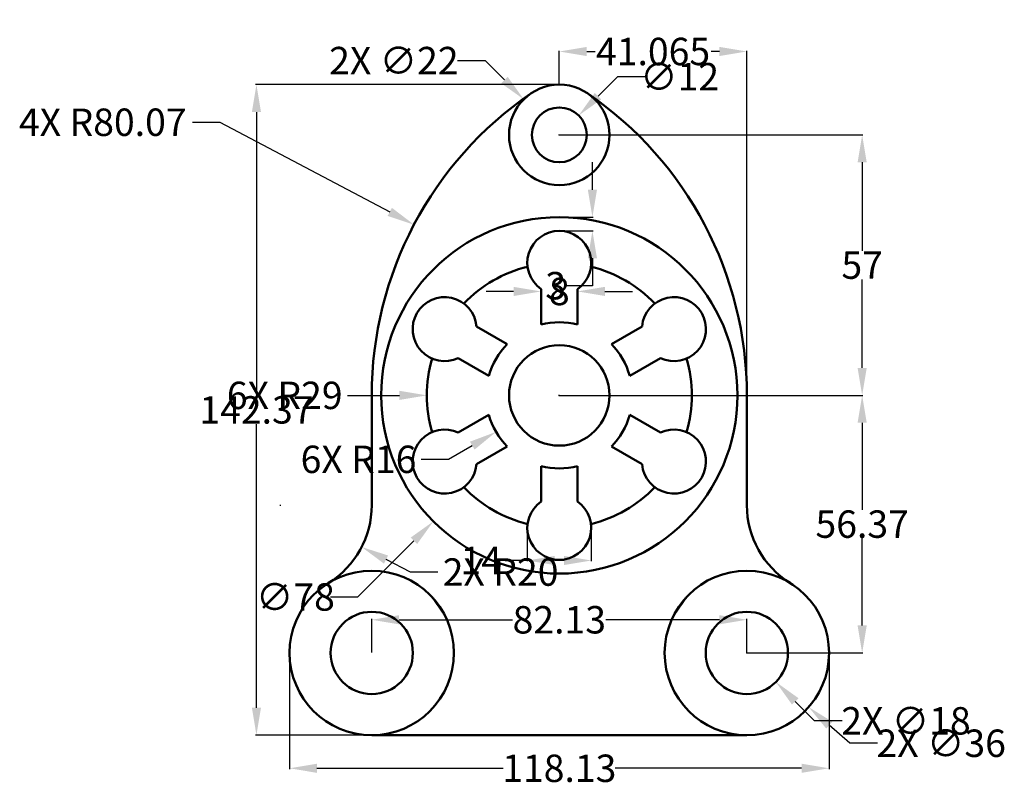
# Model space of a CAD drawing. Units: millimetres. Extents: x 708 to 923, y 97 to 265.
import ezdxf

# ---------------------------------------------------------------- set-up
doc = ezdxf.new("R2010")
doc.units = ezdxf.units.MM
doc.header["$MEASUREMENT"] = 0
doc.layers.add('M-DIMS', color=2, linetype='Continuous', lineweight=18)
doc.layers.add('M-OUTL', color=7, linetype='Continuous', lineweight=50)
doc.styles.get("Standard").update_dxf_attribs({"font": 'arial.ttf'})
doc.dimstyles.get("Standard").update_dxf_attribs({"dimtxt": 6, "dimasz": 6, "dimexe": 0.18, "dimexo": 0.0625, "dimgap": 0.09, "dimtad": 0, "dimtih": 1, "dimtoh": 1, "dimdec": 0, "dimzin": 0, "dimdsep": 46, "dimtxsty": 'Standard', "dimcen": 0.09, "dimadec": 0, "dimazin": 0, "dimtfac": 1, "dimtdec": 0, "dimtofl": 0, "dimtmove": 0, "dimatfit": 3, "dimfxl": 1, "dimtolj": 1, "dimtzin": 0, "dimarcsym": 0})

# ---------------------------------------------------------------- blocks, each defined once
blk = doc.blocks.new('*U1')
for p, q in [((-4, -10.25), (-4, -2.49)), ((4, -10.25), (4, -2.49))]:
    blk.add_line(p, q)
blk.add_arc((0, 3.25), 7, 304.8499, 235.1501)
blk = doc.blocks.new('*U2')
at = {"layer": 'M-OUTL', "color": 0, "linetype": 'ByBlock', "lineweight": -2, "transparency": 16777216}
blk.add_blockref('*U1', (825.86, 208.55), dxfattribs=at)
for p, rotation in [((803.57, 195.67), 60), ((848.16, 195.67), 300), ((803.57, 169.93), 120), ((848.16, 169.93), 240), ((825.86, 157.05), 180)]:
    blk.add_blockref('*U1', p, dxfattribs=dict(at, rotation=rotation))
blk = doc.blocks.new('MOUNTING-EAR-OD36-BORE18')
for radius in [18, 9]:
    blk.add_circle((0, 0), radius)
blk = doc.blocks.new('*D4')
at = {"layer": 'Defpoints', "color": 0, "transparency": 16777216}
for p in [(766.8, 126.44), (884.93, 126.44), (884.93, 101.19)]:
    blk.add_point(p, dxfattribs=at)
at = {"layer": 'M-DIMS', "color": 0, "lineweight": -2, "transparency": 16777216}
for p, q in [((766.8, 126.37), (766.8, 101.01)), ((884.93, 126.37), (884.93, 101.01)), ((772.8, 101.19), (813.6, 101.19)), ((878.93, 101.19), (838.13, 101.19))]:
    blk.add_line(p, q, dxfattribs=at)
at = {"layer": 'M-DIMS', "color": 0, "transparency": 16777216}
for points in [[(772.8, 102.19), (772.8, 100.19), (766.8, 101.19)], [(878.93, 102.19), (878.93, 100.19), (884.93, 101.19)]]:
    blk.add_solid(points, dxfattribs=at)
at = {"layer": 'M-DIMS', "color": 0, "transparency": 16777216, "insert": (825.86, 101.19), "char_height": 6, "attachment_point": 5}
blk.add_mtext('\\A1;118.13', dxfattribs=at)
blk = doc.blocks.new('*D5')
at = {"layer": 'Defpoints', "color": 0, "transparency": 16777216}
for p in [(759.55, 250.8), (825.86, 250.8), (784.8, 108.44)]:
    blk.add_point(p, dxfattribs=at)
at = {"layer": 'M-DIMS', "color": 0, "lineweight": -2, "transparency": 16777216}
for p, q in [((825.8, 250.8), (759.37, 250.8)), ((759.55, 244.8), (759.55, 182.77)), ((759.55, 114.44), (759.55, 176.46)), ((784.74, 108.44), (759.37, 108.44))]:
    blk.add_line(p, q, dxfattribs=at)
at = {"layer": 'M-DIMS', "color": 0, "transparency": 16777216}
for points in [[(758.55, 244.8), (760.55, 244.8), (759.55, 250.8)], [(758.55, 114.44), (760.55, 114.44), (759.55, 108.44)]]:
    blk.add_solid(points, dxfattribs=at)
at = {"layer": 'M-DIMS', "color": 0, "transparency": 16777216, "insert": (759.55, 179.62), "char_height": 6, "attachment_point": 5}
blk.add_mtext('\\A1;142.37', dxfattribs=at)
blk = doc.blocks.new('*D6')
at = {"layer": 'Defpoints', "color": 0, "transparency": 16777216}
for p in [(825.86, 182.8), (892.18, 182.8), (866.93, 126.44)]:
    blk.add_point(p, dxfattribs=at)
at = {"layer": 'M-DIMS', "color": 0, "lineweight": -2, "transparency": 16777216}
for p, q in [((825.93, 182.8), (892.36, 182.8)), ((892.18, 176.8), (892.18, 157.77)), ((892.18, 132.44), (892.18, 151.46)), ((866.99, 126.44), (892.36, 126.44))]:
    blk.add_line(p, q, dxfattribs=at)
at = {"layer": 'M-DIMS', "color": 0, "transparency": 16777216}
for points in [[(891.18, 176.8), (893.18, 176.8), (892.18, 182.8)], [(891.18, 132.44), (893.18, 132.44), (892.18, 126.44)]]:
    blk.add_solid(points, dxfattribs=at)
at = {"layer": 'M-DIMS', "color": 0, "transparency": 16777216, "insert": (892.18, 154.62), "char_height": 6, "attachment_point": 5}
blk.add_mtext('\\A1;56.37', dxfattribs=at)
blk = doc.blocks.new('*D7')
at = {"layer": 'Defpoints', "color": 0, "transparency": 16777216}
for p in [(825.86, 239.8), (892.18, 239.8), (866.93, 182.8)]:
    blk.add_point(p, dxfattribs=at)
at = {"layer": 'M-DIMS', "color": 0, "lineweight": -2, "transparency": 16777216}
for p, q in [((825.93, 239.8), (892.36, 239.8)), ((892.18, 233.8), (892.18, 214.44)), ((892.18, 188.8), (892.18, 208.16)), ((866.99, 182.8), (892.36, 182.8))]:
    blk.add_line(p, q, dxfattribs=at)
at = {"layer": 'M-DIMS', "color": 0, "transparency": 16777216}
for points in [[(891.18, 233.8), (893.18, 233.8), (892.18, 239.8)], [(891.18, 188.8), (893.18, 188.8), (892.18, 182.8)]]:
    blk.add_solid(points, dxfattribs=at)
at = {"layer": 'M-DIMS', "color": 0, "transparency": 16777216, "insert": (892.18, 211.3), "char_height": 6, "attachment_point": 5}
blk.add_mtext('\\A1;57', dxfattribs=at)
blk = doc.blocks.new('*D8')
at = {"layer": 'Defpoints', "color": 0, "transparency": 16777216}
for p in [(866.93, 133.69), (784.8, 126.44), (866.93, 126.44)]:
    blk.add_point(p, dxfattribs=at)
at = {"layer": 'M-DIMS', "color": 0, "lineweight": -2, "transparency": 16777216}
for p, q in [((784.8, 126.5), (784.8, 133.87)), ((790.8, 133.69), (815.65, 133.69)), ((860.93, 133.69), (836.08, 133.69)), ((866.93, 126.5), (866.93, 133.87))]:
    blk.add_line(p, q, dxfattribs=at)
at = {"layer": 'M-DIMS', "color": 0, "transparency": 16777216}
for points in [[(790.8, 134.69), (790.8, 132.69), (784.8, 133.69)], [(860.93, 134.69), (860.93, 132.69), (866.93, 133.69)]]:
    blk.add_solid(points, dxfattribs=at)
at = {"layer": 'M-DIMS', "color": 0, "transparency": 16777216, "insert": (825.86, 133.69), "char_height": 6, "attachment_point": 5}
blk.add_mtext('\\A1;82.13', dxfattribs=at)
blk = doc.blocks.new('*D9')
at = {"layer": 'Defpoints', "color": 0, "transparency": 16777216}
for p in [(866.93, 258.05), (825.86, 250.8), (866.93, 182.8)]:
    blk.add_point(p, dxfattribs=at)
at = {"layer": 'M-DIMS', "color": 0, "lineweight": -2, "transparency": 16777216}
for p, q in [((825.86, 250.86), (825.86, 258.23)), ((831.86, 258.05), (833.71, 258.05)), ((860.93, 258.05), (859.08, 258.05)), ((866.93, 182.86), (866.93, 258.23))]:
    blk.add_line(p, q, dxfattribs=at)
at = {"layer": 'M-DIMS', "color": 0, "transparency": 16777216}
for points in [[(831.86, 259.05), (831.86, 257.05), (825.86, 258.05)], [(860.93, 259.05), (860.93, 257.05), (866.93, 258.05)]]:
    blk.add_solid(points, dxfattribs=at)
at = {"layer": 'M-DIMS', "color": 0, "transparency": 16777216, "insert": (846.4, 258.05), "char_height": 6, "attachment_point": 5}
blk.add_mtext('\\A1;41.065', dxfattribs=at)
blk = doc.blocks.new('*D10')
at = {"layer": 'Defpoints', "color": 0, "transparency": 16777216}
for p in [(829.864092, 205.542651), (821.864092, 198.292651), (829.864092, 198.292651)]:
    blk.add_point(p, dxfattribs=at)
at = {"layer": 'M-DIMS', "color": 0, "lineweight": -2, "transparency": 16777216}
for p, q in [((815.864092, 205.542651), (809.864092, 205.542651)), ((821.864092, 198.355151), (821.864092, 205.722651)), ((829.864092, 198.355151), (829.864092, 205.722651)), ((835.864092, 205.542651), (841.864092, 205.542651))]:
    blk.add_line(p, q, dxfattribs=at)
at = {"layer": 'M-DIMS', "color": 0, "transparency": 16777216}
for points in [[(815.864092, 206.542651), (815.864092, 204.542651), (821.864092, 205.542651)], [(835.864092, 206.542651), (835.864092, 204.542651), (829.864092, 205.542651)]]:
    blk.add_solid(points, dxfattribs=at)
at = {"layer": 'M-DIMS', "color": 0, "transparency": 16777216, "insert": (825.864092, 205.542651), "char_height": 6, "attachment_point": 5}
blk.add_mtext('\\A1;8', dxfattribs=at)
blk = doc.blocks.new('*D11')
at = {"layer": 'Defpoints', "color": 0, "transparency": 16777216}
for p in [(818.86, 153.91), (832.86, 153.91), (818.86, 146.66)]:
    blk.add_point(p, dxfattribs=at)
at = {"layer": 'M-DIMS', "color": 0, "lineweight": -2, "transparency": 16777216}
for p, q in [((818.86, 153.85), (818.86, 146.48)), ((832.86, 153.85), (832.86, 146.48)), ((818.86, 146.66), (812.86, 146.66)), ((826.86, 146.66), (824.86, 146.66))]:
    blk.add_line(p, q, dxfattribs=at)
at = {"layer": 'M-DIMS', "color": 0, "transparency": 16777216}
for points in [[(824.86, 147.66), (824.86, 145.66), (818.86, 146.66)], [(826.86, 147.66), (826.86, 145.66), (832.86, 146.66)]]:
    blk.add_solid(points, dxfattribs=at)
at = {"layer": 'M-DIMS', "color": 0, "transparency": 16777216, "insert": (808.77, 146.66), "char_height": 6, "attachment_point": 5}
blk.add_mtext('\\A1;14', dxfattribs=at)
blk = doc.blocks.new('*D12')
at = {"layer": 'Defpoints', "color": 0, "transparency": 16777216}
for p in [(825.86, 221.8), (825.86, 218.8), (833.11, 218.8)]:
    blk.add_point(p, dxfattribs=at)
at = {"layer": 'M-DIMS', "color": 0, "lineweight": -2, "transparency": 16777216}
for p, q in [((833.11, 227.8), (833.11, 233.8)), ((825.93, 221.8), (833.29, 221.8)), ((825.93, 218.8), (833.29, 218.8)), ((833.11, 212.8), (833.11, 206.8)), ((833.11, 206.8), (827.11, 206.8))]:
    blk.add_line(p, q, dxfattribs=at)
at = {"layer": 'M-DIMS', "color": 0, "transparency": 16777216}
for points in [[(832.11, 227.8), (834.11, 227.8), (833.11, 221.8)], [(832.11, 212.8), (834.11, 212.8), (833.11, 218.8)]]:
    blk.add_solid(points, dxfattribs=at)
at = {"layer": 'M-DIMS', "color": 0, "transparency": 16777216, "insert": (825.06, 206.8), "char_height": 6, "attachment_point": 5}
blk.add_mtext('\\A1;3', dxfattribs=at)
blk = doc.blocks.new('*D13')
at = {"layer": 'Defpoints', "color": 0, "transparency": 16777216}
for p in [(853.39, 138.3), (880.47, 114.58)]:
    blk.add_point(p, dxfattribs=at)
at = {"layer": 'M-DIMS', "color": 0, "lineweight": -2, "transparency": 16777216}
for p, q in [((866.84, 126.44), (867.02, 126.44)), ((866.93, 126.35), (866.93, 126.53)), ((889.5, 106.67), (884.98, 110.62)), ((895.5, 106.67), (889.5, 106.67))]:
    blk.add_line(p, q, dxfattribs=at)
at = {"layer": 'M-DIMS', "color": 0, "transparency": 16777216}
blk.add_solid([(885.64, 111.38), (884.32, 109.87), (880.47, 114.58)], dxfattribs=at)
at = {"layer": 'M-DIMS', "color": 0, "transparency": 16777216, "insert": (909.48, 106.67), "char_height": 6, "attachment_point": 5}
blk.add_mtext('\\A1;2X ∅36', dxfattribs=at)
blk = doc.blocks.new('*D14')
at = {"layer": 'Defpoints', "color": 0, "transparency": 16777216}
for p in [(860.57, 132.8), (873.29, 120.07)]:
    blk.add_point(p, dxfattribs=at)
at = {"layer": 'M-DIMS', "color": 0, "lineweight": -2, "transparency": 16777216}
for p, q in [((866.84, 126.44), (867.02, 126.44)), ((866.93, 126.35), (866.93, 126.53)), ((881.77, 111.58), (877.53, 115.82)), ((887.77, 111.58), (881.77, 111.58))]:
    blk.add_line(p, q, dxfattribs=at)
at = {"layer": 'M-DIMS', "color": 0, "transparency": 16777216}
blk.add_solid([(878.24, 116.53), (876.82, 115.12), (873.29, 120.07)], dxfattribs=at)
at = {"layer": 'M-DIMS', "color": 0, "transparency": 16777216, "insert": (901.77, 111.58), "char_height": 6, "attachment_point": 5}
blk.add_mtext('\\A1;2X ∅18', dxfattribs=at)
blk = doc.blocks.new('*D15')
at = {"layer": 'Defpoints', "color": 0, "transparency": 16777216}
for p in [(830.11, 244.05), (821.62, 235.56)]:
    blk.add_point(p, dxfattribs=at)
at = {"layer": 'M-DIMS', "color": 0, "lineweight": -2, "transparency": 16777216}
for p, q in [((838.59, 252.53), (834.35, 248.29)), ((844.59, 252.53), (838.59, 252.53)), ((825.77, 239.8), (825.95, 239.8)), ((825.86, 239.71), (825.86, 239.89))]:
    blk.add_line(p, q, dxfattribs=at)
at = {"layer": 'M-DIMS', "color": 0, "transparency": 16777216}
blk.add_solid([(833.64, 249), (835.05, 247.58), (830.11, 244.05)], dxfattribs=at)
at = {"layer": 'M-DIMS', "color": 0, "transparency": 16777216, "insert": (852.21, 252.53), "char_height": 6, "attachment_point": 5}
blk.add_mtext('\\A1;∅12', dxfattribs=at)
blk = doc.blocks.new('*D16')
at = {"layer": 'Defpoints', "color": 0, "transparency": 16777216}
for p in [(818.08, 247.58), (833.64, 232.02)]:
    blk.add_point(p, dxfattribs=at)
at = {"layer": 'M-DIMS', "color": 0, "lineweight": -2, "transparency": 16777216}
for p, q in [((803.6, 256.06), (809.6, 256.06)), ((809.6, 256.06), (813.84, 251.82)), ((825.77, 239.8), (825.95, 239.8)), ((825.86, 239.71), (825.86, 239.89))]:
    blk.add_line(p, q, dxfattribs=at)
at = {"layer": 'M-DIMS', "color": 0, "transparency": 16777216}
blk.add_solid([(814.55, 252.53), (813.13, 251.11), (818.08, 247.58)], dxfattribs=at)
at = {"layer": 'M-DIMS', "color": 0, "transparency": 16777216, "insert": (789.64, 256.06), "char_height": 6, "attachment_point": 5}
blk.add_mtext('\\A1;2X ∅22', dxfattribs=at)
blk = doc.blocks.new('*D17')
at = {"layer": 'Defpoints', "color": 0, "transparency": 16777216}
for p in [(794.05, 220.15), (864.86, 182.8)]:
    blk.add_point(p, dxfattribs=at)
at = {"layer": 'M-DIMS', "color": 0, "lineweight": -2, "transparency": 16777216}
for p, q in [((745.56, 242.57), (751.56, 242.57)), ((751.56, 242.57), (788.74, 222.95)), ((864.77, 182.8), (864.95, 182.8)), ((864.86, 182.71), (864.86, 182.89))]:
    blk.add_line(p, q, dxfattribs=at)
at = {"layer": 'M-DIMS', "color": 0, "transparency": 16777216}
blk.add_solid([(789.21, 223.84), (788.27, 222.07), (794.05, 220.15)], dxfattribs=at)
at = {"layer": 'M-DIMS', "color": 0, "transparency": 16777216, "insert": (725.9, 242.57), "char_height": 6, "attachment_point": 5}
blk.add_mtext('\\A1;4X R80.07', dxfattribs=at)
blk = doc.blocks.new('*D18')
at = {"layer": 'Defpoints', "color": 0, "transparency": 16777216}
for p in [(764.8, 158.75), (782.59, 149.61)]:
    blk.add_point(p, dxfattribs=at)
at = {"layer": 'M-DIMS', "color": 0, "lineweight": -2, "transparency": 16777216}
for p, q in [((764.71, 158.75), (764.89, 158.75)), ((764.8, 158.66), (764.8, 158.84)), ((793.26, 144.13), (787.93, 146.87)), ((799.26, 144.13), (793.26, 144.13))]:
    blk.add_line(p, q, dxfattribs=at)
at = {"layer": 'M-DIMS', "color": 0, "transparency": 16777216}
blk.add_solid([(788.38, 147.76), (787.47, 145.98), (782.59, 149.61)], dxfattribs=at)
at = {"layer": 'M-DIMS', "color": 0, "transparency": 16777216, "insert": (813.01, 144.13), "char_height": 6, "attachment_point": 5}
blk.add_mtext('\\A1;2X R20', dxfattribs=at)
blk = doc.blocks.new('*D19')
at = {"layer": 'Defpoints', "color": 0, "transparency": 16777216}
for p in [(853.44, 210.38), (798.29, 155.22)]:
    blk.add_point(p, dxfattribs=at)
at = {"layer": 'M-DIMS', "color": 0, "lineweight": -2, "transparency": 16777216}
for p, q in [((825.77, 182.8), (825.95, 182.8)), ((825.86, 182.71), (825.86, 182.89)), ((781.74, 138.68), (794.04, 150.98)), ((775.74, 138.68), (781.74, 138.68))]:
    blk.add_line(p, q, dxfattribs=at)
at = {"layer": 'M-DIMS', "color": 0, "transparency": 16777216}
blk.add_solid([(793.34, 151.69), (794.75, 150.28), (798.29, 155.22)], dxfattribs=at)
at = {"layer": 'M-DIMS', "color": 0, "transparency": 16777216, "insert": (768.08, 138.68), "char_height": 6, "attachment_point": 5}
blk.add_mtext('\\A1;∅78', dxfattribs=at)
blk = doc.blocks.new('*D20')
at = {"layer": 'Defpoints', "color": 0, "transparency": 16777216}
for p in [(796.86, 182.8), (825.86, 182.8)]:
    blk.add_point(p, dxfattribs=at)
at = {"layer": 'M-DIMS', "color": 0, "lineweight": -2, "transparency": 16777216}
for p, q in [((779.46, 182.8), (790.86, 182.8)), ((825.77, 182.8), (825.95, 182.8)), ((825.86, 182.71), (825.86, 182.89))]:
    blk.add_line(p, q, dxfattribs=at)
at = {"layer": 'M-DIMS', "color": 0, "transparency": 16777216}
blk.add_solid([(790.86, 183.8), (790.86, 181.8), (796.86, 182.8)], dxfattribs=at)
at = {"layer": 'M-DIMS', "color": 0, "transparency": 16777216, "insert": (765.74, 182.8), "char_height": 6, "attachment_point": 5}
blk.add_mtext('\\A1;6X R29', dxfattribs=at)
blk = doc.blocks.new('*D21')
at = {"layer": 'Defpoints', "color": 0, "transparency": 16777216}
for p in [(825.86, 182.8), (812.01, 174.8)]:
    blk.add_point(p, dxfattribs=at)
at = {"layer": 'M-DIMS', "color": 0, "lineweight": -2, "transparency": 16777216}
for p, q in [((825.77, 182.8), (825.95, 182.8)), ((825.86, 182.71), (825.86, 182.89)), ((801.62, 168.8), (806.81, 171.8)), ((795.62, 168.8), (801.62, 168.8))]:
    blk.add_line(p, q, dxfattribs=at)
at = {"layer": 'M-DIMS', "color": 0, "transparency": 16777216}
blk.add_solid([(806.31, 172.67), (807.31, 170.93), (812.01, 174.8)], dxfattribs=at)
at = {"layer": 'M-DIMS', "color": 0, "transparency": 16777216, "insert": (781.9, 168.8), "char_height": 6, "attachment_point": 5}
blk.add_mtext('\\A1;6X R16', dxfattribs=at)

msp = doc.modelspace()

# ---------------------------------------------------------------- linework, layer by layer
at = {"layer": 'M-OUTL'}
for p, q in [((784.7989, 182.8007), (784.7989, 158.7466)), ((866.9293, 182.8007), (866.9293, 158.7466)), ((784.7989, 108.4357), (866.9293, 108.4357))]:
    msp.add_line(p, q, dxfattribs=at)
for centre, radius in [((825.8641, 239.8007), 11), ((825.8641, 239.8007), 6), ((825.8641, 182.8007), 39), ((825.8641, 182.8007), 11)]:
    msp.add_circle(centre, radius, dxfattribs=at)
for centre, radius, start, end in [((864.8641, 182.8007), 80.0652, 124.380345, 180), ((786.8641, 182.8007), 80.0652, 0, 55.619655), ((825.8641, 182.8007), 29, 103.863812, 136.136188), ((825.8641, 182.8007), 29, 43.863812, 76.136188), ((825.8641, 182.8007), 16, 75.522488, 104.477512), ((825.8641, 182.8007), 16, 135.522488, 164.477512), ((825.8641, 182.8007), 16, 15.522488, 44.477512), ((825.8641, 182.8007), 29, 163.863812, 196.136188), ((825.8641, 182.8007), 29, 343.863812, 16.136188), ((825.8641, 182.8007), 16, 195.522488, 224.477512), ((825.8641, 182.8007), 16, 315.522488, 344.477512), ((825.8641, 182.8007), 16, 255.522488, 284.477512), ((825.8641, 182.8007), 29, 223.863812, 256.136188), ((825.8641, 182.8007), 29, 283.863812, 316.136188), ((764.7989, 158.7466), 20, 301.756864, 0), ((886.9293, 158.7466), 20, 180, 238.243136), ((864.8641, 182.8007), 80.0652, 213.646297, 216.643999), ((786.8641, 182.8007), 80.0652, 323.356001, 326.353703)]:
    msp.add_arc(centre, radius, start, end, dxfattribs=at)

# ---------------------------------------------------------------- block references
for name, p in [('*U2', (0, 0)), ('MOUNTING-EAR-OD36-BORE18', (784.7989, 126.4357)), ('MOUNTING-EAR-OD36-BORE18', (866.9293, 126.4357))]:
    msp.add_blockref(name, p, dxfattribs=at)

# ---------------------------------------------------------------- dimensions: what is measured, and where the dimension line sits
at = {"layer": 'M-DIMS'}
for p1, p2, picture, middle in [((833.6447, 232.0249), (818.0835, 247.5765), '*D16', (789.6373, 256.0591)), ((853.3885, 138.2951), (880.4701, 114.5762), '*D13', (909.4843, 106.6699)), ((860.5678, 132.8021), (873.2908, 120.0692), '*D14', (901.7679, 111.5807))]:
    dim = msp.add_diameter_dim_2p(p1=p1, p2=p2, text='2X <>', dimstyle='Standard', override={"dimdec": 0, "dimlfac": 1, "dimrnd": 0, "dimzin": 0, "dimdsep": 46, "dimlunit": 2}, dxfattribs=at)
    dim.commit()
    dim.dimension.update_dxf_attribs({"geometry": picture, "text_midpoint": middle, "dimtype": 163})
for base, p1, p2, override, picture, middle in [((866.9293, 258.0507), (825.8641, 250.8007), (866.9293, 182.8007), {"dimdec": 3, "dimlfac": 1, "dimrnd": 0, "dimzin": 0, "dimdsep": 46, "dimlunit": 2}, '*D9', (846.3967, 258.0507)), ((866.9293, 133.6857), (784.7989, 126.4357), (866.9293, 126.4357), {"dimdec": 2, "dimlfac": 1, "dimrnd": 0, "dimzin": 0, "dimdsep": 46, "dimlunit": 2}, '*D8', (825.8641, 133.6857)), ((884.9293, 101.1857), (766.7989, 126.4357), (884.9293, 126.4357), {"dimdec": 2, "dimlfac": 1, "dimrnd": 0, "dimzin": 0, "dimdsep": 46, "dimlunit": 2}, '*D4', (825.8641, 101.1857))]:
    dim = msp.add_linear_dim(base=base, p1=p1, p2=p2, dimstyle='Standard', override=override, dxfattribs=at)
    dim.commit()
    dim.dimension.update_dxf_attribs({"geometry": picture, "text_midpoint": middle})
for p1, p2, picture, middle in [((821.6231, 235.5564), (830.105, 244.045), '*D15', (852.2076, 252.5337)), ((853.4424, 210.3767), (798.2857, 155.2247), '*D19', (768.0812, 138.6792))]:
    dim = msp.add_diameter_dim_2p(p1=p1, p2=p2, dimstyle='Standard', override={"dimdec": 0, "dimlfac": 1, "dimrnd": 0, "dimzin": 0, "dimdsep": 46, "dimlunit": 2}, dxfattribs=at)
    dim.commit()
    dim.dimension.update_dxf_attribs({"geometry": picture, "text_midpoint": middle, "dimtype": 163})
for center, mpoint, text, override, picture, middle in [((864.8641, 182.8007), (794.0462, 220.1539), '4X <>', {"dimdec": 2, "dimlfac": 1, "dimrnd": 0, "dimzin": 0, "dimdsep": 46, "dimlunit": 2}, '*D17', (725.9041, 242.5658)), ((825.8641, 182.8007), (796.8641, 182.801), '6X <>', {"dimdec": 0, "dimlfac": 1, "dimrnd": 0, "dimzin": 0, "dimdsep": 46, "dimlunit": 2}, '*D20', (779.4641, 182.8012)), ((764.7989, 158.7466), (782.5891, 149.6083), '2X <>', {"dimdec": 0, "dimlfac": 1, "dimrnd": 0, "dimzin": 0, "dimdsep": 46, "dimlunit": 2}, '*D18', (813.0088, 144.1253))]:
    dim = msp.add_radius_dim(center=center, mpoint=mpoint, text=text, dimstyle='Standard', override=override, dxfattribs=at)
    dim.commit()
    dim.dimension.update_dxf_attribs({"geometry": picture, "text_midpoint": middle, "dimtype": 164})
for base, p1, p2, angle, override, picture, middle in [((759.54891, 250.80072), (784.7989, 108.43566), (825.86409, 250.80072), 90, {"dimdec": 2, "dimlfac": 1, "dimrnd": 0, "dimzin": 0, "dimdsep": 46, "dimlunit": 2}, '*D5', (759.54891, 179.61819)), ((892.1793, 239.8007), (866.9293, 182.8007), (825.8641, 239.8007), 90, {"dimdec": 0, "dimlfac": 1, "dimrnd": 0, "dimzin": 0, "dimdsep": 46, "dimlunit": 2}, '*D7', (892.1793, 211.3007)), ((833.1141, 218.8007), (825.8641, 221.8007), (825.8641, 218.8007), 270, {"dimdec": 0, "dimlfac": 1, "dimrnd": 0, "dimzin": 0, "dimdsep": 46, "dimlunit": 2}, '*D12', (825.0596, 206.8007)), ((829.8641, 205.5427), (821.8641, 198.2927), (829.8641, 198.2927), 0, {"dimdec": 0, "dimlfac": 1, "dimrnd": 0, "dimzin": 0, "dimdsep": 46, "dimlunit": 2}, '*D10', (825.8641, 205.5427)), ((892.17928, 182.80072), (866.92928, 126.43566), (825.86409, 182.80072), 90, {"dimdec": 2, "dimlfac": 1, "dimrnd": 0, "dimzin": 0, "dimdsep": 46, "dimlunit": 2}, '*D6', (892.17928, 154.61819)), ((818.8645, 146.665), (832.8637, 153.915), (818.8645, 153.915), 180, {"dimdec": 0, "dimlfac": 1, "dimrnd": 0, "dimzin": 0, "dimdsep": 46, "dimlunit": 2}, '*D11', (808.7718, 146.665))]:
    dim = msp.add_linear_dim(base=base, p1=p1, p2=p2, angle=angle, dimstyle='Standard', override=override, dxfattribs=at)
    dim.commit()
    dim.dimension.update_dxf_attribs({"geometry": picture, "text_midpoint": middle})
dim = msp.add_radius_dim(center=(825.8641, 182.8007), mpoint=(812.0076, 174.8008), text='6X <>', dimstyle='Standard', override={"dimdec": 0, "dimlfac": 1, "dimrnd": 0, "dimzin": 0, "dimdsep": 46, "dimlunit": 2}, dxfattribs=at)
dim.commit()
dim.dimension.update_dxf_attribs({"geometry": '*D21', "text_midpoint": (781.8964, 168.8009)})

doc.saveas('drawing.dxf')
